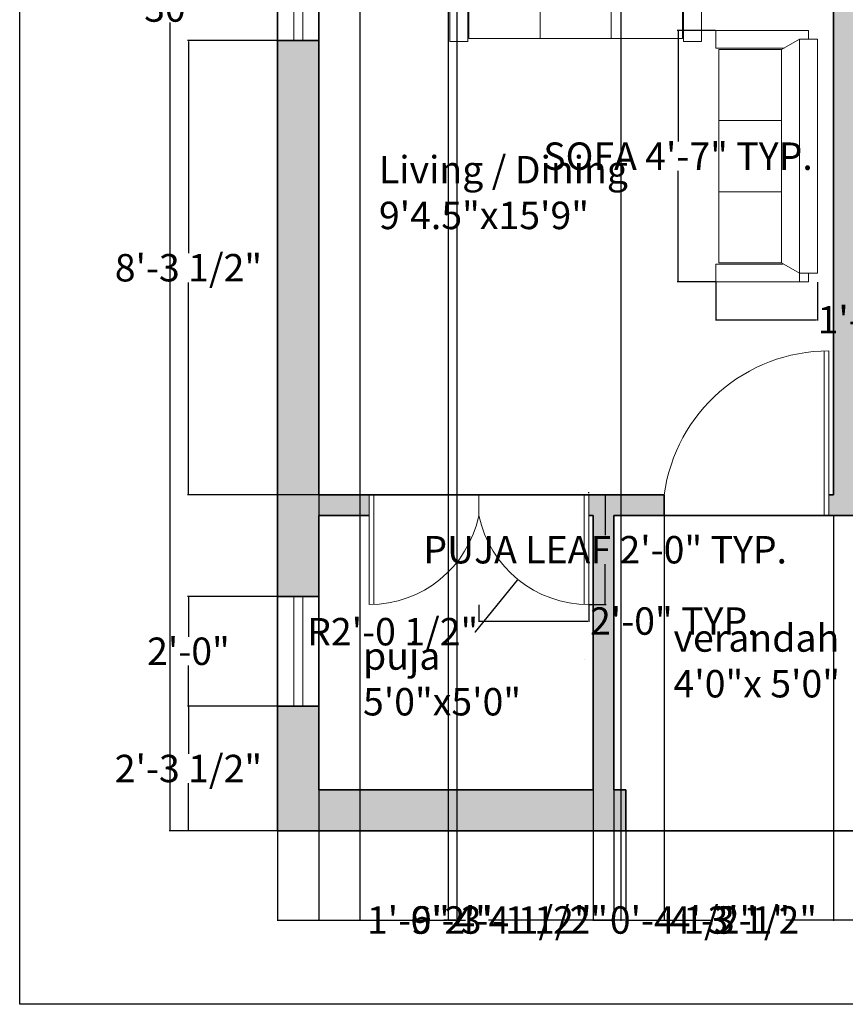
# Model space of a CAD drawing. Units: inches. Extents: x 335 to 688, y 1043 to 1486.
# Tile 1 of 7: x 335 to 515, y 1043 to 1258. Entities that reach past the tile are written whole.
import ezdxf

# ---------------------------------------------------------------- set-up
doc = ezdxf.new("R2010")
doc.units = ezdxf.units.IN
doc.header["$MEASUREMENT"] = 0
for name, color, linetype, lineweight in [('A-ANNO-DIMS', 2, 'Continuous', 18), ('A-ANNO-TTLB', 7, 'Continuous', 25), ('A-AREA-IDEN', 7, 'Continuous', 18), ('A-DOOR', 4, 'Continuous', 18), ('A-FURN', 8, 'Continuous', 18), ('A-GLAZ', 4, 'Continuous', 18), ('A-WALL', 7, 'Continuous', 35), ('A-WALL-PATT', 252, 'Continuous', 13)]:
    doc.layers.add(name, color=color, linetype=linetype, lineweight=lineweight)
doc.styles.get("Standard").update_dxf_attribs({"font": 'arial.ttf'})
doc.dimstyles.get("Standard").update_dxf_attribs({"dimtxt": 6, "dimasz": 0.18, "dimexe": 0.18, "dimexo": 0.0625, "dimgap": 0.09, "dimtad": 0, "dimtih": 1, "dimtoh": 1, "dimdec": 1, "dimzin": 0, "dimdsep": 46, "dimlunit": 3, "dimtxsty": 'Standard', "dimcen": 0.09, "dimadec": 0, "dimazin": 0, "dimtfac": 1, "dimtdec": 1, "dimtofl": 0, "dimtmove": 0, "dimatfit": 3, "dimfxl": 1, "dimtolj": 1, "dimtzin": 0, "dimarcsym": 0})

# ---------------------------------------------------------------- blocks, each defined once
blk = doc.blocks.new('*D4')
at = {"layer": 'A-ANNO-DIMS', "color": 0, "lineweight": -2, "transparency": 16777216}
for p, q in [((391.04, 1440.97), (367.42, 1440.97)), ((367.6, 1440.79), (367.6, 1264.12)), ((367.6, 1081.15), (367.6, 1257.81)), ((391.04, 1080.97), (367.42, 1080.97))]:
    blk.add_line(p, q, dxfattribs=at)
at = {"layer": 'A-ANNO-DIMS', "color": 0, "transparency": 16777216}
for points in [[(367.57, 1440.79), (367.63, 1440.79), (367.6, 1440.97)], [(367.57, 1081.15), (367.63, 1081.15), (367.6, 1080.97)]]:
    blk.add_solid(points, dxfattribs=at)
at = {"layer": 'Defpoints', "color": 0, "transparency": 16777216}
for p in [(391.11, 1440.97), (367.6, 1080.97), (391.11, 1080.97)]:
    blk.add_point(p, dxfattribs=at)
at = {"layer": 'A-ANNO-DIMS', "color": 0, "transparency": 16777216, "insert": (367.6, 1260.97), "char_height": 6, "attachment_point": 5}
blk.add_mtext("\\A1;30'", dxfattribs=at)
blk = doc.blocks.new('SOFA-THREE-SEAT')
for p, q in [((53.08, 22.23), (1.96, 22.23)), ((1.96, 18.31), (1.96, 22.23)), ((53.08, 18.31), (53.08, 22.23)), ((0, 20.27), (0, 0)), ((1.96, 20.27), (0, 20.27)), ((55.04, 20.27), (53.08, 20.27)), ((55.04, 20.27), (55.04, 0)), ((55.04, 18.31), (1.96, 18.31)), ((4.17, 14.38), (1.96, 18.31)), ((53.08, 18.31), (50.88, 14.38)), ((3.92, 14.94), (3.92, 0)), ((19.74, 0.65), (19.74, 14.38)), ((35.3, 0.65), (35.3, 14.38)), ((50.87, 0.65), (50.87, 14.38)), ((51.12, 14.69), (51.12, 0)), ((3.92, 0), (0, 0)), ((51.12, 0), (55.04, 0))]:
    blk.add_line(p, q)
blk.add_lwpolyline([(50.88, 14.38), (4.17, 14.38), (4.17, 0.65), (50.87, 0.65)])
blk = doc.blocks.new('WIN-60IN')
for p, q in [((0, 0), (0, 60)), ((3.5, 0), (3.5, 60)), ((5.5, 60), (5.5, 0)), ((9, 60), (9, 0))]:
    blk.add_line(p, q)
blk = doc.blocks.new('DOOR-36IN')
for p, q in [((0, 36), (36, 36)), ((36, 35), (0, 35))]:
    blk.add_line(p, q)
blk.add_arc((-0.32, 36), 36.32, 277.6281, 0)
blk = doc.blocks.new('DOOR-24IN-LEAF')
for p, q in [((23, 0), (23, 24)), ((24, 24), (24, 0))]:
    blk.add_line(p, q)
blk.add_arc((24, 24.52), 24.52, 191.8123, 270)
blk = doc.blocks.new('*D19')
at = {"layer": 'A-ANNO-DIMS', "color": 0, "lineweight": -2, "transparency": 16777216}
for p, q in [((486.83, 1256.08), (478.45, 1256.08)), ((478.63, 1255.9), (478.63, 1231.75)), ((478.63, 1201.22), (478.63, 1225.36)), ((486.83, 1201.04), (478.45, 1201.04))]:
    blk.add_line(p, q, dxfattribs=at)
at = {"layer": 'A-ANNO-DIMS', "color": 0, "transparency": 16777216}
for points in [[(478.6, 1255.9), (478.66, 1255.9), (478.63, 1256.08)], [(478.6, 1201.22), (478.66, 1201.22), (478.63, 1201.04)]]:
    blk.add_solid(points, dxfattribs=at)
at = {"layer": 'Defpoints', "color": 0, "transparency": 16777216}
for p in [(486.89, 1256.08), (478.63, 1201.04), (486.89, 1201.04)]:
    blk.add_point(p, dxfattribs=at)
at = {"layer": 'A-ANNO-DIMS', "color": 0, "transparency": 16777216, "insert": (478.63, 1228.56), "char_height": 6, "attachment_point": 5}
blk.add_mtext('\\A1;SOFA 4\'-7" TYP.', dxfattribs=at)
blk = doc.blocks.new('*D20')
at = {"layer": 'A-ANNO-DIMS', "color": 0, "lineweight": -2, "transparency": 16777216}
for p, q in [((486.89, 1200.97), (486.89, 1192.6)), ((509.12, 1200.97), (509.12, 1192.6)), ((487.07, 1192.78), (508.94, 1192.78)), ((509.12, 1192.78), (509.3, 1192.78))]:
    blk.add_line(p, q, dxfattribs=at)
at = {"layer": 'A-ANNO-DIMS', "color": 0, "transparency": 16777216}
for points in [[(487.07, 1192.81), (487.07, 1192.75), (486.89, 1192.78)], [(508.94, 1192.81), (508.94, 1192.75), (509.12, 1192.78)]]:
    blk.add_solid(points, dxfattribs=at)
at = {"layer": 'Defpoints', "color": 0, "transparency": 16777216}
for p in [(486.89, 1201.04), (509.12, 1201.04), (509.12, 1192.78)]:
    blk.add_point(p, dxfattribs=at)
at = {"layer": 'A-ANNO-DIMS', "color": 0, "transparency": 16777216, "insert": (529.72, 1192.78), "char_height": 6, "attachment_point": 5}
blk.add_mtext('\\A1;1\'-10" TYP.', dxfattribs=at)
blk = doc.blocks.new('*D33')
at = {"layer": 'A-ANNO-DIMS', "color": 0, "lineweight": -2, "transparency": 16777216}
for p, q in [((459.17, 1154.47), (462.89, 1154.47)), ((462.71, 1154.29), (462.71, 1145.62)), ((462.71, 1130.65), (462.71, 1139.31)), ((459.17, 1130.47), (462.89, 1130.47))]:
    blk.add_line(p, q, dxfattribs=at)
at = {"layer": 'A-ANNO-DIMS', "color": 0, "transparency": 16777216}
for points in [[(462.68, 1154.29), (462.74, 1154.29), (462.71, 1154.47)], [(462.68, 1130.65), (462.74, 1130.65), (462.71, 1130.47)]]:
    blk.add_solid(points, dxfattribs=at)
at = {"layer": 'Defpoints', "color": 0, "transparency": 16777216}
for p in [(459.11, 1154.47), (462.71, 1154.47), (459.11, 1130.47)]:
    blk.add_point(p, dxfattribs=at)
at = {"layer": 'A-ANNO-DIMS', "color": 0, "transparency": 16777216, "insert": (462.71, 1142.47), "char_height": 6, "attachment_point": 5}
blk.add_mtext('\\A1;PUJA LEAF 2\'-0" TYP.', dxfattribs=at)
blk = doc.blocks.new('*D34')
at = {"layer": 'A-ANNO-DIMS', "color": 0, "lineweight": -2, "transparency": 16777216}
for p, q in [((435.11, 1130.4), (435.11, 1126.69)), ((459.11, 1130.4), (459.11, 1126.69)), ((435.29, 1126.87), (458.93, 1126.87)), ((459.11, 1126.87), (459.29, 1126.87))]:
    blk.add_line(p, q, dxfattribs=at)
at = {"layer": 'A-ANNO-DIMS', "color": 0, "transparency": 16777216}
for points in [[(435.29, 1126.9), (435.29, 1126.84), (435.11, 1126.87)], [(458.93, 1126.9), (458.93, 1126.84), (459.11, 1126.87)]]:
    blk.add_solid(points, dxfattribs=at)
at = {"layer": 'Defpoints', "color": 0, "transparency": 16777216}
for p in [(435.11, 1130.47), (459.11, 1130.47), (459.11, 1126.87)]:
    blk.add_point(p, dxfattribs=at)
at = {"layer": 'A-ANNO-DIMS', "color": 0, "transparency": 16777216, "insert": (477.71, 1126.87), "char_height": 6, "attachment_point": 5}
blk.add_mtext('\\A1;2\'-0" TYP.', dxfattribs=at)
blk = doc.blocks.new('*D39')
at = {"layer": 'A-ANNO-DIMS', "color": 0, "lineweight": -2, "transparency": 16777216}
for p, q in [((409.09, 1289), (409.09, 1061.29)), ((430.25, 1289), (430.25, 1061.29)), ((409.27, 1061.47), (411.89, 1061.47)), ((430.07, 1061.47), (427.45, 1061.47))]:
    blk.add_line(p, q, dxfattribs=at)
at = {"layer": 'A-ANNO-DIMS', "color": 0, "transparency": 16777216}
for points in [[(409.27, 1061.5), (409.27, 1061.44), (409.09, 1061.47)], [(430.07, 1061.5), (430.07, 1061.44), (430.25, 1061.47)]]:
    blk.add_solid(points, dxfattribs=at)
at = {"layer": 'Defpoints', "color": 0, "transparency": 16777216}
for p in [(409.09, 1289.07), (430.25, 1289.07), (430.25, 1061.47)]:
    blk.add_point(p, dxfattribs=at)
at = {"layer": 'A-ANNO-DIMS', "color": 0, "transparency": 16777216, "insert": (419.67, 1061.47), "char_height": 6, "attachment_point": 5}
blk.add_mtext('\\A1;1\'-9"', dxfattribs=at)
blk = doc.blocks.new('*D44')
at = {"layer": 'A-ANNO-DIMS', "color": 0, "lineweight": -2, "transparency": 16777216}
for p, q in [((460.11, 1089.9), (460.11, 1061.29)), ((464.61, 1089.9), (464.61, 1061.29)), ((460.29, 1061.47), (464.43, 1061.47)), ((464.61, 1061.47), (464.79, 1061.47))]:
    blk.add_line(p, q, dxfattribs=at)
at = {"layer": 'A-ANNO-DIMS', "color": 0, "transparency": 16777216}
for points in [[(460.29, 1061.5), (460.29, 1061.44), (460.11, 1061.47)], [(464.43, 1061.5), (464.43, 1061.44), (464.61, 1061.47)]]:
    blk.add_solid(points, dxfattribs=at)
at = {"layer": 'Defpoints', "color": 0, "transparency": 16777216}
for p in [(460.11, 1089.97), (464.61, 1089.97), (464.61, 1061.47)]:
    blk.add_point(p, dxfattribs=at)
at = {"layer": 'A-ANNO-DIMS', "color": 0, "transparency": 16777216, "insert": (479.84, 1061.47), "char_height": 6, "attachment_point": 5}
blk.add_mtext('\\A1;0\'-4 1/2"', dxfattribs=at)
blk = doc.blocks.new('*D45')
at = {"layer": 'A-ANNO-DIMS', "color": 0, "lineweight": -2, "transparency": 16777216}
for p, q in [((475.61, 1149.9), (475.61, 1061.29)), ((512.61, 1149.9), (512.61, 1061.29)), ((475.79, 1061.47), (486.04, 1061.47)), ((512.43, 1061.47), (502.17, 1061.47))]:
    blk.add_line(p, q, dxfattribs=at)
at = {"layer": 'A-ANNO-DIMS', "color": 0, "transparency": 16777216}
for points in [[(475.79, 1061.5), (475.79, 1061.44), (475.61, 1061.47)], [(512.43, 1061.5), (512.43, 1061.44), (512.61, 1061.47)]]:
    blk.add_solid(points, dxfattribs=at)
at = {"layer": 'Defpoints', "color": 0, "transparency": 16777216}
for p in [(475.61, 1149.97), (512.61, 1149.97), (512.61, 1061.47)]:
    blk.add_point(p, dxfattribs=at)
at = {"layer": 'A-ANNO-DIMS', "color": 0, "transparency": 16777216, "insert": (494.11, 1061.47), "char_height": 6, "attachment_point": 5}
blk.add_mtext('\\A1;3\'-1"', dxfattribs=at)
blk = doc.blocks.new('*D46')
at = {"layer": 'A-ANNO-DIMS', "color": 0, "lineweight": -2, "transparency": 16777216}
for p, q in [((391.04, 1132.26), (371.43, 1132.26)), ((371.61, 1132.08), (371.61, 1123.42)), ((371.61, 1108.44), (371.61, 1117.11)), ((391.04, 1108.26), (371.43, 1108.26))]:
    blk.add_line(p, q, dxfattribs=at)
at = {"layer": 'A-ANNO-DIMS', "color": 0, "transparency": 16777216}
for points in [[(371.58, 1132.08), (371.64, 1132.08), (371.61, 1132.26)], [(371.58, 1108.44), (371.64, 1108.44), (371.61, 1108.26)]]:
    blk.add_solid(points, dxfattribs=at)
at = {"layer": 'Defpoints', "color": 0, "transparency": 16777216}
for p in [(371.61, 1132.26), (391.11, 1132.26), (391.11, 1108.26)]:
    blk.add_point(p, dxfattribs=at)
at = {"layer": 'A-ANNO-DIMS', "color": 0, "transparency": 16777216, "insert": (371.61, 1120.26), "char_height": 6, "attachment_point": 5}
blk.add_mtext('\\A1;2\'-0"', dxfattribs=at)
blk = doc.blocks.new('*D48')
at = {"layer": 'A-ANNO-DIMS', "color": 0, "lineweight": -2, "transparency": 16777216}
for p, q in [((391.04, 1108.26), (371.43, 1108.26)), ((371.61, 1108.08), (371.61, 1097.81)), ((371.61, 1081.15), (371.61, 1091.42)), ((391.04, 1080.97), (371.43, 1080.97))]:
    blk.add_line(p, q, dxfattribs=at)
at = {"layer": 'A-ANNO-DIMS', "color": 0, "transparency": 16777216}
for points in [[(371.58, 1108.08), (371.64, 1108.08), (371.61, 1108.26)], [(371.58, 1081.15), (371.64, 1081.15), (371.61, 1080.97)]]:
    blk.add_solid(points, dxfattribs=at)
at = {"layer": 'Defpoints', "color": 0, "transparency": 16777216}
for p in [(371.61, 1108.26), (391.11, 1108.26), (391.11, 1080.97)]:
    blk.add_point(p, dxfattribs=at)
at = {"layer": 'A-ANNO-DIMS', "color": 0, "transparency": 16777216, "insert": (371.61, 1094.61), "char_height": 6, "attachment_point": 5}
blk.add_mtext('\\A1;2\'-3 1/2"', dxfattribs=at)
blk = doc.blocks.new('*D49')
at = {"layer": 'A-ANNO-DIMS', "color": 0, "lineweight": -2, "transparency": 16777216}
for p, q in [((400.04, 1253.85), (371.43, 1253.85)), ((371.61, 1253.67), (371.61, 1207.35)), ((371.61, 1154.65), (371.61, 1200.96)), ((400.04, 1154.47), (371.43, 1154.47))]:
    blk.add_line(p, q, dxfattribs=at)
at = {"layer": 'A-ANNO-DIMS', "color": 0, "transparency": 16777216}
for points in [[(371.58, 1253.67), (371.64, 1253.67), (371.61, 1253.85)], [(371.58, 1154.65), (371.64, 1154.65), (371.61, 1154.47)]]:
    blk.add_solid(points, dxfattribs=at)
at = {"layer": 'Defpoints', "color": 0, "transparency": 16777216}
for p in [(371.61, 1253.85), (400.11, 1253.85), (400.11, 1154.47)]:
    blk.add_point(p, dxfattribs=at)
at = {"layer": 'A-ANNO-DIMS', "color": 0, "transparency": 16777216, "insert": (371.61, 1204.16), "char_height": 6, "attachment_point": 5}
blk.add_mtext('\\A1;8\'-3 1/2"', dxfattribs=at)
blk = doc.blocks.new('*D55')
at = {"layer": 'A-ANNO-DIMS', "color": 0, "lineweight": -2, "transparency": 16777216}
for p, q in [((391.11, 1080.9), (391.11, 1061.29)), ((467.19, 1080.9), (467.19, 1061.29)), ((391.29, 1061.47), (421.06, 1061.47)), ((467.01, 1061.47), (437.23, 1061.47))]:
    blk.add_line(p, q, dxfattribs=at)
at = {"layer": 'A-ANNO-DIMS', "color": 0, "transparency": 16777216}
for points in [[(391.29, 1061.5), (391.29, 1061.44), (391.11, 1061.47)], [(467.01, 1061.5), (467.01, 1061.44), (467.19, 1061.47)]]:
    blk.add_solid(points, dxfattribs=at)
at = {"layer": 'Defpoints', "color": 0, "transparency": 16777216}
for p in [(391.11, 1080.97), (467.19, 1080.97), (467.19, 1061.47)]:
    blk.add_point(p, dxfattribs=at)
at = {"layer": 'A-ANNO-DIMS', "color": 0, "transparency": 16777216, "insert": (429.15, 1061.47), "char_height": 6, "attachment_point": 5}
blk.add_mtext('\\A1;6\'-4"', dxfattribs=at)
blk = doc.blocks.new('*D56')
at = {"layer": 'A-ANNO-DIMS', "color": 0, "lineweight": -2, "transparency": 16777216}
for p, q in [((467.19, 1080.9), (467.19, 1061.29)), ((518.67, 1080.9), (518.67, 1061.29)), ((467.37, 1061.47), (477.75, 1061.47)), ((518.49, 1061.47), (508.1, 1061.47))]:
    blk.add_line(p, q, dxfattribs=at)
at = {"layer": 'A-ANNO-DIMS', "color": 0, "transparency": 16777216}
for points in [[(467.37, 1061.5), (467.37, 1061.44), (467.19, 1061.47)], [(518.49, 1061.5), (518.49, 1061.44), (518.67, 1061.47)]]:
    blk.add_solid(points, dxfattribs=at)
at = {"layer": 'Defpoints', "color": 0, "transparency": 16777216}
for p in [(467.19, 1080.97), (518.67, 1080.97), (518.67, 1061.47)]:
    blk.add_point(p, dxfattribs=at)
at = {"layer": 'A-ANNO-DIMS', "color": 0, "transparency": 16777216, "insert": (492.93, 1061.47), "char_height": 6, "attachment_point": 5}
blk.add_mtext('\\A1;4\'-3 1/2"', dxfattribs=at)
blk = doc.blocks.new('*D60')
at = {"layer": 'A-ANNO-DIMS', "color": 0, "lineweight": -2, "transparency": 16777216}
for p, q in [((400.11, 1343.4), (400.11, 1061.29)), ((428.36, 1343.4), (428.36, 1061.29)), ((400.29, 1061.47), (428.18, 1061.47)), ((428.36, 1061.47), (428.54, 1061.47))]:
    blk.add_line(p, q, dxfattribs=at)
at = {"layer": 'A-ANNO-DIMS', "color": 0, "transparency": 16777216}
for points in [[(400.29, 1061.5), (400.29, 1061.44), (400.11, 1061.47)], [(428.18, 1061.5), (428.18, 1061.44), (428.36, 1061.47)]]:
    blk.add_solid(points, dxfattribs=at)
at = {"layer": 'Defpoints', "color": 0, "transparency": 16777216}
for p in [(400.11, 1343.47), (428.36, 1343.47), (428.36, 1061.47)]:
    blk.add_point(p, dxfattribs=at)
at = {"layer": 'A-ANNO-DIMS', "color": 0, "transparency": 16777216, "insert": (443.65, 1061.47), "char_height": 6, "attachment_point": 5}
blk.add_mtext('\\A1;2\'-4 1/2"', dxfattribs=at)
blk = doc.blocks.new('*D61')
at = {"layer": 'A-ANNO-DIMS', "color": 0, "lineweight": -2, "transparency": 16777216}
for p, q in [((428.36, 1347.9), (428.36, 1061.29)), ((466.11, 1347.9), (466.11, 1061.29)), ((428.54, 1061.47), (432.18, 1061.47)), ((465.93, 1061.47), (462.29, 1061.47))]:
    blk.add_line(p, q, dxfattribs=at)
at = {"layer": 'A-ANNO-DIMS', "color": 0, "transparency": 16777216}
for points in [[(428.54, 1061.5), (428.54, 1061.44), (428.36, 1061.47)], [(465.93, 1061.5), (465.93, 1061.44), (466.11, 1061.47)]]:
    blk.add_solid(points, dxfattribs=at)
at = {"layer": 'Defpoints', "color": 0, "transparency": 16777216}
for p in [(428.36, 1347.97), (466.11, 1347.97), (466.11, 1061.47)]:
    blk.add_point(p, dxfattribs=at)
at = {"layer": 'A-ANNO-DIMS', "color": 0, "transparency": 16777216, "insert": (447.24, 1061.47), "char_height": 6, "attachment_point": 5}
blk.add_mtext('\\A1;3\'-1 1/2"', dxfattribs=at)
blk = doc.blocks.new('*D67')
at = {"layer": 'A-ANNO-DIMS', "color": 0, "lineweight": -2, "transparency": 16777216}
for p, q in [((459.02, 1154.99), (459.2, 1154.99)), ((459.11, 1154.9), (459.11, 1155.08)), ((434.37, 1124.54), (443.53, 1135.82)), ((434.19, 1124.54), (434.37, 1124.54))]:
    blk.add_line(p, q, dxfattribs=at)
at = {"layer": 'A-ANNO-DIMS', "color": 0, "transparency": 16777216}
blk.add_solid([(443.51, 1135.84), (443.55, 1135.8), (443.65, 1135.96)], dxfattribs=at)
at = {"layer": 'Defpoints', "color": 0, "transparency": 16777216}
for p in [(459.11, 1154.99), (443.65, 1135.96)]:
    blk.add_point(p, dxfattribs=at)
at = {"layer": 'A-ANNO-DIMS', "color": 0, "transparency": 16777216, "insert": (416.26, 1124.54), "char_height": 6, "attachment_point": 5}
blk.add_mtext('\\A1;R2\'-0 1/2"', dxfattribs=at)

msp = doc.modelspace()

# ---------------------------------------------------------------- hatches: boundary and pattern name
at = {"layer": 'A-WALL-PATT'}
h = msp.add_hatch(color=256, dxfattribs=at)
h.dxf.hatch_style = 1
h.paths.add_polyline_path([(478.71, 1440.97), (391.11, 1440.97), (391.11, 1411.42), (400.11, 1411.42), (400.11, 1431.97), (466.11, 1431.97), (466.11, 1347.97), (466.11, 1343.47), (470.61, 1343.47), (470.61, 1367.47), (512.61, 1367.47), (512.61, 1350.97), (517.11, 1350.97), (517.11, 1372.97), (512.61, 1372.97), (512.61, 1371.97), (470.61, 1371.97), (470.61, 1431.97), (478.71, 1431.97)])
h.paths.add_polyline_path([(631.11, 1440.97), (502.71, 1440.97), (502.71, 1431.97), (512.61, 1431.97), (512.61, 1404.97), (517.11, 1404.97), (517.11, 1431.97), (622.11, 1431.97), (622.11, 1401.6), (631.11, 1401.6)])
h.paths.add_polyline_path([(631.11, 1341.6), (622.11, 1341.6), (622.11, 1313.47), (517.11, 1313.47), (517.11, 1314.47), (512.61, 1314.47), (512.61, 1313.47), (512.61, 1307.97), (517.11, 1307.97), (517.11, 1308.97), (553.11, 1308.97), (553.11, 1262.47), (558.61, 1262.47), (558.61, 1266.97), (557.61, 1266.97), (557.61, 1308.97), (622.11, 1308.97), (622.11, 1297.63), (631.11, 1297.63)])
h.paths.add_polyline_path([(631.11, 1273.63), (622.11, 1273.63), (622.11, 1266.97), (590.61, 1266.97), (590.61, 1262.47), (622.11, 1262.47), (622.11, 1230.86), (631.11, 1230.86)])
h.paths.add_polyline_path([(400.11, 1253.85), (391.11, 1253.85), (391.11, 1132.26), (400.11, 1132.26), (400.11, 1149.97), (411.11, 1149.97), (411.11, 1154.47), (400.11, 1154.47)], flags=17)
h.paths.add_polyline_path([(400.11, 1375.42), (391.11, 1375.42), (391.11, 1313.85), (400.11, 1313.85), (400.11, 1343.47), (428.36, 1343.47), (428.36, 1347.97), (400.11, 1347.97)])
h = msp.add_hatch(color=256, dxfattribs=at)
h.dxf.hatch_style = 1
h.paths.add_polyline_path([(467.19, 1089.97), (464.61, 1089.97), (464.61, 1149.97), (475.61, 1149.97), (475.61, 1154.47), (459.11, 1154.47), (459.11, 1149.97), (460.11, 1149.97), (460.11, 1089.97), (400.11, 1089.97), (400.11, 1108.26), (391.11, 1108.26), (391.11, 1080.97), (467.19, 1080.97)])
h.paths.add_polyline_path([(631.11, 1170.86), (622.11, 1170.86), (622.11, 1154.47), (517.11, 1154.47), (517.11, 1271.97), (512.61, 1271.97), (512.61, 1154.47), (511.61, 1154.47), (511.61, 1149.97), (512.61, 1149.97), (622.11, 1149.97), (622.11, 1089.97), (518.67, 1089.97), (518.67, 1080.97), (631.11, 1080.97)])

# ---------------------------------------------------------------- linework, layer by layer
at = {"layer": 'A-ANNO-TTLB'}
msp.add_lwpolyline([(334.72, 1486.4), (681.01, 1486.4), (681.01, 1043.03), (334.72, 1043.03)], close=True, dxfattribs=at)
at = {"layer": 'A-DOOR'}
for p, q in [((511.61, 1185.97), (511.61, 1149.97)), ((411.11, 1154.47), (411.11, 1130.47)), ((435.11, 1154.47), (435.11, 1149.97)), ((459.11, 1130.47), (459.11, 1154.47)), ((511.61, 1149.97), (475.61, 1149.97)), ((512.61, 1149.97), (511.61, 1149.97)), ((458.11, 1118.47), (458.11, 1118.48))]:
    msp.add_line(p, q, dxfattribs=at)
at = {"layer": 'A-GLAZ'}
for p, q in [((391.11, 1108.26), (391.11, 1132.26)), ((394.61, 1108.26), (394.61, 1132.26)), ((396.61, 1132.26), (396.61, 1108.26)), ((400.11, 1132.26), (400.11, 1108.26))]:
    msp.add_line(p, q, dxfattribs=at)
at = {"layer": 'A-WALL'}
for p, q in [((391.11, 1440.97), (391.11, 1080.97)), ((400.11, 1343.47), (400.11, 1154.47)), ((512.61, 1271.97), (512.61, 1154.47)), ((400.11, 1253.85), (391.11, 1253.85)), ((400.11, 1154.47), (475.61, 1154.47)), ((475.61, 1149.97), (475.61, 1154.47)), ((511.61, 1154.47), (512.61, 1154.47)), ((400.11, 1149.97), (411.11, 1149.97)), ((400.11, 1149.97), (400.11, 1089.97)), ((459.11, 1149.97), (460.11, 1149.97)), ((460.11, 1149.97), (460.11, 1089.97)), ((464.61, 1149.97), (464.61, 1089.97)), ((464.61, 1149.97), (622.11, 1149.97)), ((391.11, 1132.26), (400.11, 1132.26)), ((400.11, 1108.26), (391.11, 1108.26)), ((391.11, 1108.26), (391.11, 1108.26)), ((400.11, 1089.97), (460.11, 1089.97)), ((464.61, 1089.97), (467.19, 1089.97)), ((467.19, 1080.97), (467.19, 1089.97)), ((391.11, 1080.97), (631.11, 1080.97)), ((518.67, 1080.97), (467.19, 1080.97))]:
    msp.add_line(p, q, dxfattribs=at)

# ---------------------------------------------------------------- block references
at = {"layer": 'A-DOOR', "extrusion": (0, 0, -1), "zscale": -1, "rotation": 90.00000000000087}
msp.add_blockref('DOOR-36IN', (-475.61, 1149.97), dxfattribs=at)
at = {"layer": 'A-DOOR', "extrusion": (0, 0, -1), "zscale": -1}
msp.add_blockref('DOOR-24IN-LEAF', (-435.11, 1130.47), dxfattribs=at)
at = {"layer": 'A-DOOR'}
msp.add_blockref('DOOR-24IN-LEAF', (435.11, 1130.47), dxfattribs=at)
at = {"layer": 'A-FURN'}
msp.add_blockref('SOFA-THREE-SEAT', (428.73, 1253.66), dxfattribs=at)
at = {"layer": 'A-FURN', "rotation": 269.9999999999972}
msp.add_blockref('SOFA-THREE-SEAT', (486.89, 1256.08), dxfattribs=at)
at = {"layer": 'A-GLAZ'}
msp.add_blockref('WIN-60IN', (391.11, 1253.85), dxfattribs=at)

# ---------------------------------------------------------------- texts
at = {"layer": 'A-AREA-IDEN', "char_height": 6, "attachment_point": 1}
for s, width, insert in [('Living / Dining\\P9\'4.5"x15\'9"', 56.0083, (413.25, 1228.6)), ('verandah \\P4\'0"x 5\'0"', 58.4428, (477.65, 1126.16)), ('puja \\P5\'0"x5\'0"', 37.4564, (409.77, 1122.22))]:
    msp.add_mtext_dynamic_manual_height_columns(s, width=width, gutter_width=1, heights=[0], dxfattribs=dict(at, insert=insert))

# ---------------------------------------------------------------- dimensions: what is measured, and where the dimension line sits
at = {"layer": 'A-ANNO-DIMS'}
for base, p1, p2, override, picture, middle in [((367.6, 1080.97), (391.11, 1440.97), (391.11, 1080.97), {"dimclrd": 0, "dimclre": 0, "dimclrt": 0}, '*D4', (367.6, 1260.97)), ((371.61, 1253.85), (400.11, 1154.47), (400.11, 1253.85), {"dimdec": 1, "dimlfac": 1, "dimrnd": 0, "dimzin": 1, "dimdsep": 46, "dimlunit": 4, "dimfrac": 2}, '*D49', (371.61, 1204.16)), ((371.61, 1132.26), (391.11, 1108.26), (391.11, 1132.26), {"dimdec": 1, "dimlfac": 1, "dimrnd": 0, "dimzin": 1, "dimdsep": 46, "dimlunit": 4, "dimfrac": 2}, '*D46', (371.61, 1120.26)), ((371.61, 1108.26), (391.11, 1080.97), (391.11, 1108.26), {"dimdec": 1, "dimlfac": 1, "dimrnd": 0, "dimzin": 1, "dimdsep": 46, "dimlunit": 4, "dimfrac": 2}, '*D48', (371.61, 1094.61))]:
    dim = msp.add_linear_dim(base=base, p1=p1, p2=p2, angle=90, dimstyle='Standard', override=override, dxfattribs=at)
    dim.commit()
    dim.dimension.update_dxf_attribs({"geometry": picture, "text_midpoint": middle})
for base, p1, p2, picture, middle in [((466.1064, 1061.4667), (428.3646, 1347.9667), (466.1064, 1347.9667), '*D61', (447.2355, 1061.4667)), ((428.3646, 1061.4667), (400.1064, 1343.4667), (428.3646, 1343.4667), '*D60', (443.651, 1061.4667)), ((430.25, 1061.47), (409.09, 1289.07), (430.25, 1289.07), '*D39', (419.67, 1061.47)), ((512.61, 1061.47), (475.61, 1149.97), (512.61, 1149.97), '*D45', (494.11, 1061.47)), ((464.61, 1061.47), (460.11, 1089.97), (464.61, 1089.97), '*D44', (479.84, 1061.47)), ((467.19, 1061.47), (391.11, 1080.97), (467.19, 1080.97), '*D55', (429.15, 1061.47)), ((518.67, 1061.47), (467.19, 1080.97), (518.67, 1080.97), '*D56', (492.93, 1061.47))]:
    dim = msp.add_linear_dim(base=base, p1=p1, p2=p2, dimstyle='Standard', override={"dimdec": 1, "dimlfac": 1, "dimrnd": 0, "dimzin": 1, "dimdsep": 46, "dimlunit": 4, "dimfrac": 2}, dxfattribs=at)
    dim.commit()
    dim.dimension.update_dxf_attribs({"geometry": picture, "text_midpoint": middle})
for base, p1, p2, angle, text, picture, middle in [((478.63, 1201.04), (486.89, 1256.08), (486.89, 1201.04), 270, 'SOFA <> TYP.', '*D19', (478.63, 1228.56)), ((462.71, 1154.47), (459.11, 1130.47), (459.11, 1154.47), 90, 'PUJA LEAF <> TYP.', '*D33', (462.71, 1142.47))]:
    dim = msp.add_linear_dim(base=base, p1=p1, p2=p2, angle=angle, text=text, dimstyle='Standard', override={"dimdec": 1, "dimlfac": 1, "dimrnd": 0, "dimzin": 1, "dimdsep": 46, "dimlunit": 4, "dimfrac": 2}, dxfattribs=at)
    dim.commit()
    dim.dimension.update_dxf_attribs({"geometry": picture, "text_midpoint": middle})
for base, p1, p2, picture, middle in [((509.12, 1192.78), (486.89, 1201.04), (509.12, 1201.04), '*D20', (529.72, 1192.78)), ((459.11, 1126.87), (435.11, 1130.47), (459.11, 1130.47), '*D34', (477.71, 1126.87))]:
    dim = msp.add_linear_dim(base=base, p1=p1, p2=p2, text='<> TYP.', dimstyle='Standard', override={"dimdec": 1, "dimlfac": 1, "dimrnd": 0, "dimzin": 1, "dimdsep": 46, "dimlunit": 4, "dimfrac": 2}, dxfattribs=at)
    dim.commit()
    dim.dimension.update_dxf_attribs({"geometry": picture, "text_midpoint": middle})
dim = msp.add_radius_dim(center=(459.11, 1154.99), mpoint=(443.65, 1135.96), dimstyle='Standard', override={"dimdec": 1, "dimlfac": 1, "dimrnd": 0, "dimzin": 1, "dimdsep": 46, "dimlunit": 4, "dimfrac": 2}, dxfattribs=at)
dim.commit()
dim.dimension.update_dxf_attribs({"geometry": '*D67', "text_midpoint": (416.26, 1124.54), "dimtype": 164})

doc.saveas('drawing.dxf')
